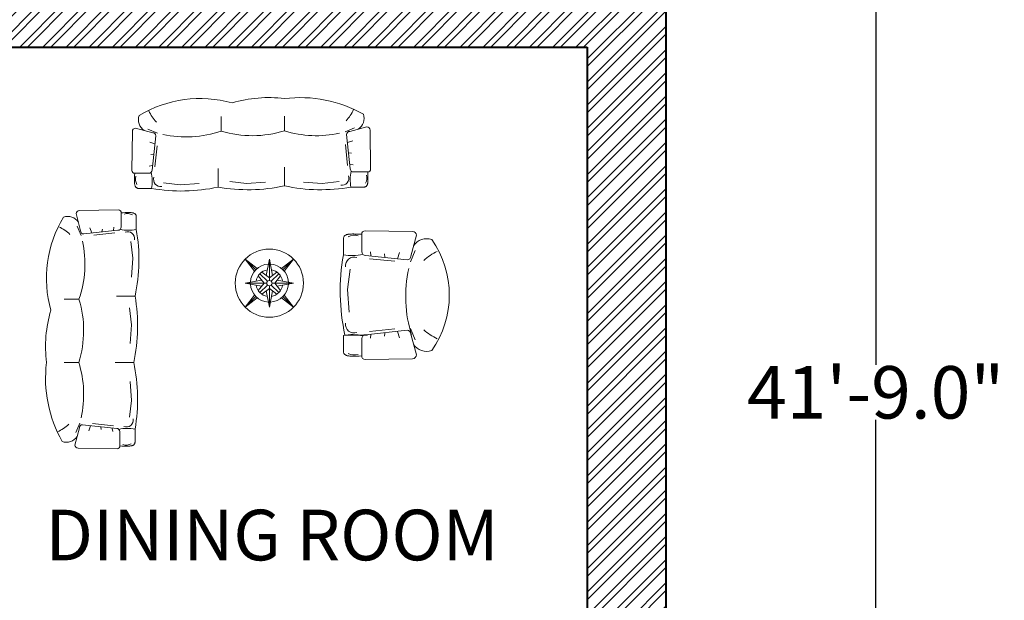
# Model space of a CAD drawing. Units: inches. Extents: x 528 to 2520, y -151 to 1354.
# Tile 9 of 41: x 812 to 924, y 1043 to 1109. Entities that reach past the tile are written whole.
import ezdxf

# ---------------------------------------------------------------- set-up
doc = ezdxf.new("R2010")
doc.units = ezdxf.units.IN
doc.header["$MEASUREMENT"] = 0
for name, color, linetype, lineweight in [('A-ANNO-DIMS', 2, 'Continuous', 18), ('A-AREA-IDEN', 7, 'Continuous', 18), ('A-FURN', 8, 'Continuous', 18), ('A-WALL-PATT', 6, 'Continuous', 13), ('walls', 7, 'Continuous', 40)]:
    doc.layers.add(name, color=color, linetype=linetype, lineweight=lineweight)
doc.styles.get("Standard").update_dxf_attribs({"font": 'arial.ttf'})
doc.dimstyles.get("Standard").update_dxf_attribs({"dimtxt": 6, "dimasz": 2, "dimexe": 0.18, "dimexo": 0.0625, "dimgap": 0.09, "dimtad": 0, "dimtih": 1, "dimtoh": 1, "dimdec": 1, "dimzin": 0, "dimdsep": 46, "dimlunit": 3, "dimtxsty": 'Standard', "dimblk": 'ARCHTICK', "dimcen": 0.09, "dimadec": 0, "dimazin": 0, "dimtfac": 1, "dimtdec": 1, "dimtofl": 0, "dimtmove": 0, "dimatfit": 3, "dimfxl": 1, "dimtolj": 1, "dimtzin": 0, "dimarcsym": 0})

# ---------------------------------------------------------------- blocks, each defined once
blk = doc.blocks.new('floor')
for p, q in [((-9.45, 11.55), (-18.9, 18.9)), ((-18.9, 18.9), (-10.55, 10.55)), ((-18.9, 18.9), (-11.55, 9.45)), ((0, 18.9), (-2.39, 6.06)), ((2.39, 6.06), (0, 18.9)), ((0, 18.9), (0, 2.1)), ((18.9, 18.9), (9.45, 11.55)), ((18.9, 18.9), (10.55, 10.55)), ((11.55, 9.45), (18.9, 18.9)), ((0, 4.2), (-5.83, 8.73)), ((5.83, 8.73), (0, 4.2)), ((-6.06, 2.39), (-18.9, 0)), ((-18.9, 0), (-6.06, -2.39)), ((-18.9, 0), (-2.1, 0)), ((-8.73, 5.83), (-4.2, 0)), ((-7.42, 7.42), (-1.48, 1.48)), ((7.42, 7.42), (1.48, 1.48)), ((2.1, 0), (18.9, 0)), ((4.2, 0), (8.73, 5.83)), ((18.9, 0), (6.06, 2.39)), ((6.06, -2.39), (18.9, 0)), ((-4.2, 0), (-8.73, -5.83)), ((-1.48, -1.48), (-7.42, -7.42)), ((-5.83, -8.73), (0, -4.2)), ((-2.39, -6.06), (0, -18.9)), ((0, -2.1), (0, -18.9)), ((0, -4.2), (5.83, -8.73)), ((0, -18.9), (2.39, -6.06)), ((1.48, -1.48), (7.42, -7.42)), ((8.73, -5.83), (4.2, 0)), ((-11.55, -9.45), (-18.9, -18.9)), ((-10.55, -10.55), (-18.9, -18.9)), ((-18.9, -18.9), (-9.45, -11.55)), ((9.45, -11.55), (18.9, -18.9)), ((10.55, -10.55), (18.9, -18.9)), ((18.9, -18.9), (11.55, -9.45))]:
    blk.add_line(p, q)
for radius in [26.73, 2.1]:
    blk.add_circle((0, 0), radius)
for radius, start, end in [(14.92, 92.86089, 177.13911), (10.5, 98.70166, 171.29834), (14.92, 2.86089, 87.13911), (10.5, 8.70166, 81.29834), (14.92, 182.86089, 267.13911), (10.5, 188.70166, 261.29834), (14.92, 272.86089, 357.13911), (10.5, 278.70166, 351.29834)]:
    blk.add_arc((0, 0), radius, start, end)
blk = doc.blocks.new('3-s')
for p, q in [((-3099.98, -914.27), (-3099.98, -918.75)), ((-3086.85, -913.54), (-3099.1, -913.37)), ((-3104.73, -915.45), (-3104.73, -919.55)), ((-3087.27, -919.9), (-3085.85, -914.54)), ((-3098.98, -919.75), (-3088.27, -920.9)), ((-3097.59, -919.77), (-3097.73, -918.83)), ((-3093.97, -920.17), (-3094.1, -919.37)), ((-3090.75, -920.58), (-3090.21, -918.96)), ((-3086.18, -918.42), (-3087.39, -921.38)), ((-3102.96, -923.27), (-3103.63, -928.52)), ((-3091.42, -921.25), (-3098, -920.58)), ((-3103.63, -928.52), (-3103.23, -934.44)), ((-3104.33, -940.39), (-3098.51, -940.39)), ((-3087.08, -940.39), (-3082.49, -940.39)), ((-3103.63, -952.27), (-3103.23, -946.35)), ((-3102.96, -957.52), (-3103.63, -952.27)), ((-3087.15, -960.23), (-3082.56, -960.23)), ((-3104.73, -961.23), (-3098.92, -961.23)), ((-3104.04, -973.11), (-3103.63, -967.19)), ((-3103.37, -978.36), (-3104.04, -973.11)), ((-3105.14, -986.18), (-3105.14, -982.07)), ((-3091.82, -980.37), (-3098.4, -981.05)), ((-3098, -981.85), (-3098.13, -982.8)), ((-3094.37, -981.45), (-3094.51, -982.26)), ((-3091.15, -981.05), (-3090.61, -982.66)), ((-3086.59, -983.2), (-3087.79, -980.24))]:
    blk.add_line(p, q)
for points in [[(-3099.98, -914.27), (-3100.65, -914.23), (-3101.21, -914.21), (-3101.68, -914.19), (-3102.07, -914.18), (-3102.4, -914.18), (-3102.68, -914.19), (-3102.91, -914.21), (-3103.11, -914.22), (-3103.29, -914.24), (-3103.46, -914.26), (-3103.62, -914.29), (-3103.76, -914.33), (-3103.89, -914.36), (-3104.01, -914.41), (-3104.12, -914.47), (-3104.23, -914.53), (-3104.33, -914.6), (-3104.43, -914.69), (-3104.51, -914.78), (-3104.58, -914.89), (-3104.65, -915.01), (-3104.69, -915.14), (-3104.72, -915.29), (-3104.73, -915.45)], [(-3100.39, -987.35), (-3101.05, -987.39), (-3101.61, -987.42), (-3102.08, -987.43), (-3102.48, -987.44), (-3102.81, -987.44), (-3103.08, -987.43), (-3103.31, -987.42), (-3103.51, -987.4), (-3103.7, -987.38), (-3103.87, -987.36), (-3104.02, -987.33), (-3104.16, -987.3), (-3104.29, -987.26), (-3104.41, -987.21), (-3104.53, -987.16), (-3104.63, -987.09), (-3104.73, -987.02), (-3104.83, -986.94), (-3104.91, -986.84), (-3104.99, -986.73), (-3105.05, -986.61), (-3105.1, -986.48), (-3105.13, -986.34), (-3105.14, -986.18)]]:
    blk.add_lwpolyline(points)
blk.add_lwpolyline([(-3087.67, -981.72), (-3086.25, -987.09, -0.414214), (-3087.25, -988.09), (-3099.51, -988.25, -0.464301), (-3100.39, -987.35), (-3100.39, -982.87, -0.414214), (-3099.39, -981.87), (-3088.67, -980.72, -0.414214)], format="xyb", close=True)
for centre, radius, start, end in [((-3099.16, -914.2), 0.826, 85.8896, 185.5116), ((-3086.85, -914.54), 1, 0, 90), ((-3101.91, -917.78), 3.27, 72.9324, 119.1125), ((-3083.18, -919.47), 4.05, 71.0879, 146.7483), ((-3117.09, -935.46), 40.42, 352.9967, 29.3731), ((-3051.57, -928.95), 53.99, 169.9808, 192.2408), ((-3102.44, -907.13), 12.63, 259.551, 282.5683), ((-3101.95, -922.43), 2.24, 70.9224, 187.7848), ((-3098.98, -918.75), 1, 180, 270), ((-3088.27, -919.9), 1, 270, 0), ((-3074.56, -931.19), 13.81, 115.1439, 132.7066), ((-3055.23, -930.36), 33.39, 167.467, 197.4804), ((-3051.57, -951.84), 53.99, 167.7592, 190.0192), ((-3055.23, -950.42), 33.39, 162.5196, 197.0763), ((-3117.09, -945.32), 40.42, 343.5213, 7.0033), ((-3114.19, -966.81), 37.23, 329.0051, 15.6244), ((-3055.63, -971.26), 33.39, 160.7021, 192.533), ((-3051.97, -972.68), 53.99, 167.7592, 190.0192), ((-3102.35, -979.2), 2.24, 172.2152, 289.0776), ((-3102.84, -994.5), 12.63, 77.4317, 100.449), ((-3074.97, -970.43), 13.81, 227.2934, 244.8561), ((-3083.58, -982.16), 4.05, 213.2517, 288.9121), ((-3102.31, -983.84), 3.27, 240.8875, 287.0676)]:
    blk.add_arc(centre, radius, start, end)
blk = doc.blocks.new('si-s')
for p, q in [((-3100.11, -942.03), (-3112.37, -941.87)), ((-3118, -943.94), (-3118, -948.05)), ((-3113.25, -942.77), (-3113.25, -947.25)), ((-3100.54, -948.4), (-3099.11, -943.03)), ((-3110.86, -948.27), (-3110.99, -947.32)), ((-3104.01, -949.07), (-3103.48, -947.46)), ((-3099.45, -946.92), (-3100.66, -949.88)), ((-3112.25, -948.25), (-3101.54, -949.4)), ((-3104.68, -949.75), (-3111.26, -949.07)), ((-3107.24, -948.67), (-3107.37, -947.86)), ((-3116.23, -951.76), (-3116.9, -957.01)), ((-3116.9, -957.01), (-3116.5, -962.93)), ((-3112.25, -968.73), (-3101.54, -967.58)), ((-3104.68, -967.23), (-3111.26, -967.9)), ((-3104.01, -967.9), (-3103.48, -969.52)), ((-3099.45, -970.06), (-3100.66, -967.1)), ((-3118, -973.03), (-3118, -968.93)), ((-3117.6, -968.89), (-3111.78, -968.89)), ((-3113.25, -974.21), (-3113.25, -969.73)), ((-3110.86, -968.71), (-3110.99, -969.65)), ((-3107.24, -968.31), (-3107.37, -969.11)), ((-3100.54, -968.58), (-3099.11, -973.94)), ((-3100.11, -974.94), (-3112.37, -975.11))]:
    blk.add_line(p, q)
for points in [[(-3113.25, -942.77), (-3113.92, -942.73), (-3114.48, -942.7), (-3114.95, -942.69), (-3115.34, -942.68), (-3115.67, -942.68), (-3115.94, -942.69), (-3116.18, -942.7), (-3116.38, -942.72), (-3116.56, -942.74), (-3116.73, -942.76), (-3116.88, -942.79), (-3117.03, -942.82), (-3117.16, -942.86), (-3117.28, -942.91), (-3117.39, -942.96), (-3117.5, -943.02), (-3117.6, -943.1), (-3117.69, -943.18), (-3117.78, -943.28), (-3117.85, -943.39), (-3117.91, -943.51), (-3117.96, -943.64), (-3117.99, -943.78), (-3118, -943.94)], [(-3113.25, -974.21), (-3113.92, -974.25), (-3114.48, -974.27), (-3114.95, -974.29), (-3115.34, -974.3), (-3115.67, -974.3), (-3115.94, -974.29), (-3116.18, -974.28), (-3116.38, -974.26), (-3116.56, -974.24), (-3116.73, -974.22), (-3116.88, -974.19), (-3117.03, -974.16), (-3117.16, -974.12), (-3117.28, -974.07), (-3117.39, -974.02), (-3117.5, -973.95), (-3117.6, -973.88), (-3117.69, -973.79), (-3117.78, -973.7), (-3117.85, -973.59), (-3117.91, -973.47), (-3117.96, -973.34), (-3117.99, -973.19), (-3118, -973.03)]]:
    blk.add_lwpolyline(points)
for centre, radius, start, end in [((-3112.43, -942.69), 0.826, 85.8896, 185.5116), ((-3100.11, -943.03), 1, 0, 90), ((-3115.18, -946.28), 3.27, 72.9324, 119.1125), ((-3096.45, -947.96), 4.05, 71.0879, 146.7483), ((-3115.55, -958.49), 24.96, 324.8902, 35.1098), ((-3112.25, -947.25), 1, 180, 270), ((-3087.83, -959.69), 13.81, 115.1439, 132.7066), ((-3064.84, -957.44), 53.99, 169.9808, 192.2408), ((-3115.71, -935.62), 12.63, 259.551, 282.5683), ((-3115.22, -950.92), 2.24, 70.9224, 187.7848), ((-3101.54, -948.4), 1, 270, 0), ((-3068.5, -958.86), 33.39, 167.467, 197.4804), ((-3115.22, -966.05), 2.24, 172.2152, 289.0776), ((-3101.54, -968.58), 1, 0, 90), ((-3087.83, -957.29), 13.81, 227.2934, 244.8561), ((-3115.71, -981.35), 12.63, 77.4317, 100.449), ((-3112.25, -969.73), 1, 90, 180), ((-3096.45, -969.01), 4.05, 213.2517, 288.9121), ((-3115.18, -970.7), 3.27, 240.8875, 287.0676), ((-3112.43, -974.29), 0.826, 174.4884, 274.1104), ((-3100.11, -973.94), 1, 270, 0)]:
    blk.add_arc(centre, radius, start, end)
blk = doc.blocks.new('_ArchTick')
at = {"color": 0, "linetype": 'ByBlock', "const_width": 0.15}
blk.add_lwpolyline([(-0.5, -0.5), (0.5, 0.5)], dxfattribs=at)
blk = doc.blocks.new('*D24')
at = {"layer": 'A-ANNO-DIMS', "color": 0, "lineweight": -2, "transparency": 16777216}
for p, q in [((885.76, 1317.1), (909.9, 1317.1)), ((909.72, 1317.1), (909.72, 1069.76)), ((909.72, 816.1), (909.72, 1063.45)), ((885.76, 816.1), (909.9, 816.1))]:
    blk.add_line(p, q, dxfattribs=at)
at = {"layer": 'Defpoints', "color": 0, "transparency": 16777216}
for p in [(885.7, 1317.1), (885.7, 816.1), (909.72, 816.1)]:
    blk.add_point(p, dxfattribs=at)
at = {"layer": 'A-ANNO-DIMS', "color": 0, "lineweight": -2, "transparency": 16777216, "xscale": 2, "yscale": 2, "zscale": 2}
for p, rotation in [((909.72, 1317.1), 90), ((909.72, 816.1), 270)]:
    blk.add_blockref('_ArchTick', p, dxfattribs=dict(at, rotation=rotation))
at = {"layer": 'A-ANNO-DIMS', "color": 0, "transparency": 16777216, "insert": (909.72, 1066.6), "char_height": 6, "attachment_point": 5}
blk.add_mtext('\\A1;41\'-9.0"', dxfattribs=at)

msp = doc.modelspace()

# ---------------------------------------------------------------- hatches: boundary and pattern name
at = {"layer": 'A-WALL-PATT'}
h = msp.add_hatch(dxfattribs=at)
h.set_pattern_fill('ANSI32', color=256, scale=5)
h.paths.add_polyline_path([(595.7, 1163.86), (586.7, 1163.86), (586.7, 969.1), (598.24, 969.1), (603.24, 969.1), (603.24, 974.1), (595.7, 974.1), (595.7, 1082.1), (691.7, 1082.1), (691.7, 1087.1), (691.7, 1106.1), (697.7, 1106.1), (697.7, 1111.1), (686.7, 1111.1), (686.7, 1087.1), (595.7, 1087.1)])
h.paths.add_polyline_path([(688.7, 974.1), (651.24, 974.1), (651.24, 969.1), (688.7, 969.1)])
h.paths.add_polyline_path([(885.7, 1171.37), (876.7, 1171.37), (876.7, 1111.1), (786.7, 1111.1), (786.7, 1106.1), (876.7, 1106.1), (876.7, 974.1), (786.7, 974.1), (786.7, 969.1), (876.7, 969.1), (876.7, 825.1), (834.7, 825.1), (834.7, 816.1), (885.7, 816.1)])
h.paths.add_polyline_path([(885.7, 1317.1), (876.65, 1317.1), (876.65, 1308.1), (876.7, 1308.1), (876.7, 1248.1), (822.7, 1248.1), (822.7, 1243.1), (876.7, 1243.1), (876.7, 1219.37), (885.7, 1219.37)])
h.paths.add_polyline_path([(852.65, 1317.1), (787.7, 1317.1), (787.7, 1248.1), (784.26, 1248.1), (784.26, 1243.1), (792.7, 1243.1), (792.7, 1249.1), (792.7, 1308.1), (852.65, 1308.1)])
h.paths.add_polyline_path([(684.7, 1317.1), (619.7, 1317.1), (619.7, 1308.1), (679.7, 1308.1), (679.7, 1248.1), (679.7, 1243.1), (684.7, 1243.1), (684.7, 1248.25)])
h.paths.add_polyline_path([(595.7, 1308.1), (595.7, 1317.1), (586.7, 1317.1), (586.7, 1211.86), (595.7, 1211.86), (595.7, 1243.1), (649.7, 1243.1), (649.7, 1248.1), (595.7, 1248.1)])
h.paths.add_polyline_path([(744.7, 969.1), (744.7, 974.1), (724.7, 974.1), (724.7, 969.1), (739.7, 969.1), (739.7, 874.29), (744.7, 874.29)])
h.paths.add_polyline_path([(739.7, 969.1), (727.7, 969.1), (727.7, 965.12), (730.74, 965.12), (730.74, 961.68), (734.43, 961.68), (734.43, 957.24), (739.7, 957.24)], flags=17)
h.paths.add_polyline_path([(786.7, 825.1), (744.7, 825.1), (744.7, 832.29), (739.7, 832.29), (739.7, 816.1), (786.7, 816.1)])

# ---------------------------------------------------------------- linework, layer by layer
at = {"layer": 'walls'}
for p, q in [((885.7, 1317.1), (885.7, 816.1)), ((786.7, 1106.1), (876.7, 1106.1)), ((876.7, 1106.1), (876.7, 974.1))]:
    msp.add_line(p, q, dxfattribs=at)

# ---------------------------------------------------------------- block references
at = {"layer": 'A-FURN'}
for p, xscale, yscale, zscale, rotation in [((1185.13, 2222.75), -0.3648213827119744, 0.3648213827119744, 0.3648213827119362, 270), ((-307.72, 726.93), 0.3648213827118212, 0.3648213827118212, 0.3648213827118212, 180)]:
    msp.add_blockref('3-s', p, dxfattribs=dict(at, xscale=xscale, yscale=yscale, zscale=zscale, rotation=rotation))
for name, p, xscale, yscale, zscale in [('si-s', (2227.75, 1501.62), 0.4422535540881025, 0.4422535540881025, 0.4422535540881025), ('floor', (840.33, 1079.09, -157.77), 0.1459285530847694, 0.1459285530847694, 0.1459285530847694)]:
    msp.add_blockref(name, p, dxfattribs=dict(at, xscale=xscale, yscale=yscale, zscale=zscale))

# ---------------------------------------------------------------- texts
at = {"layer": 'A-AREA-IDEN'}
msp.add_text('DINING ROOM', height=5.7926, dxfattribs=at).set_placement((814.71, 1047.38))

# ---------------------------------------------------------------- dimensions: what is measured, and where the dimension line sits
at = {"layer": 'A-ANNO-DIMS'}
dim = msp.add_linear_dim(base=(909.72, 816.1), p1=(885.7, 1317.1), p2=(885.7, 816.1), angle=90, dimstyle='Standard', override={"dimclrd": 0, "dimclre": 0, "dimclrt": 0}, dxfattribs=at)
dim.commit()
dim.dimension.update_dxf_attribs({"geometry": '*D24', "text_midpoint": (909.72, 1066.6)})

doc.saveas('drawing.dxf')
